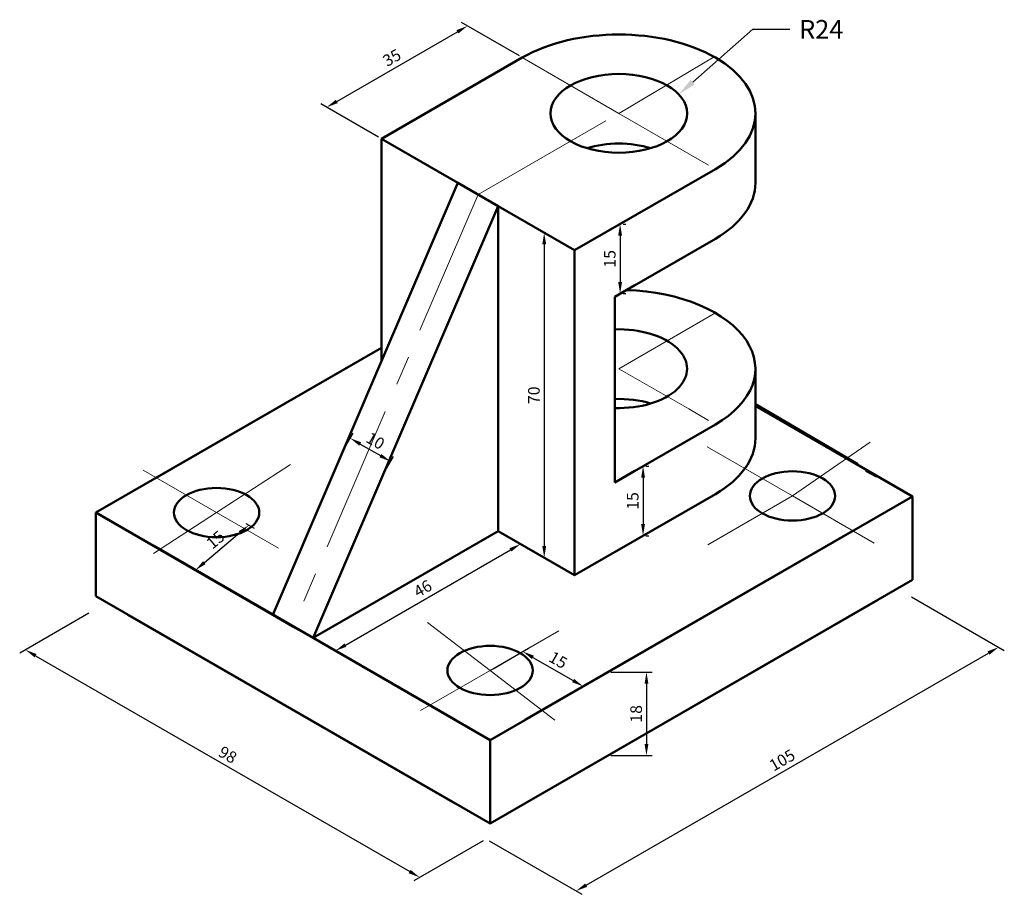
# Model space of a CAD drawing. Units: millimetres. Extents: x 3049 to 3261, y 1454 to 1642.
import ezdxf
from ezdxf import colors
from ezdxf.entities.mleader import LeaderData, LeaderLine
from ezdxf.math import Vec2, Vec3

# ---------------------------------------------------------------- set-up
doc = ezdxf.new("R2010")
doc.units = ezdxf.units.MM
doc.linetypes.add('CENTER', pattern=[50.8, 31.75, -6.35, 6.35, -6.35])
for name, color, linetype, lineweight in [('M-CNTR', 4, 'CENTER', 18), ('M-DIMS', 2, 'Continuous', 25), ('M-OUTL', 7, 'Continuous', 50)]:
    doc.layers.add(name, color=color, linetype=linetype, lineweight=lineweight)
doc.styles.get("Standard").update_dxf_attribs({"font": 'arial.ttf'})
doc.dimstyles.new('ISO-25', dxfattribs={"dimtxt": 2.5, "dimasz": 2.5, "dimexe": 1.25, "dimexo": 0.625, "dimtad": 1, "dimtxsty": 'Standard', "dimcen": 2.5, "dimadec": 0, "dimazin": 0, "dimtfac": 1, "dimtmove": 0, "dimatfit": 3, "dimfxl": 1, "dimarcsym": 0})

# ---------------------------------------------------------------- blocks, each defined once
blk = doc.blocks.new('*D1')
at = {"layer": 'Defpoints', "color": 0, "transparency": 16777216}
for p in [(3240.3, 1518.12), (3259.67, 1506.94), (3149.37, 1465.62)]:
    blk.add_point(p, dxfattribs=at)
at = {"layer": 'M-DIMS', "color": 0, "lineweight": -2, "transparency": 16777216}
for p, q in [((3240.93, 1517.76), (3260.92, 1506.22)), ((3170.91, 1455.69), (3257.51, 1505.69)), ((3149.99, 1465.26), (3169.99, 1453.72))]:
    blk.add_line(p, q, dxfattribs=at)
at = {"layer": 'M-DIMS', "color": 0, "transparency": 16777216}
for points in [[(3257.3, 1506.05), (3257.72, 1505.33), (3259.67, 1506.94)], [(3170.7, 1456.05), (3171.11, 1455.33), (3168.74, 1454.44)]]:
    blk.add_solid(points, dxfattribs=at)
at = {"layer": 'M-DIMS', "color": 0, "transparency": 16777216, "insert": (3213.26, 1482.34), "char_height": 2.5, "attachment_point": 5, "rotation": 30}
blk.add_mtext('105', dxfattribs=at)
blk = doc.blocks.new('*D2')
at = {"layer": 'Defpoints', "color": 0, "transparency": 16777216}
for p in [(3064.5, 1514.62), (3149.37, 1465.62), (3135.07, 1457.37)]:
    blk.add_point(p, dxfattribs=at)
at = {"layer": 'M-DIMS', "color": 0, "lineweight": -2, "transparency": 16777216}
for p, q in [((3063.87, 1514.26), (3048.95, 1505.65)), ((3052.37, 1505.12), (3132.91, 1458.62)), ((3148.74, 1465.26), (3133.82, 1456.65))]:
    blk.add_line(p, q, dxfattribs=at)
at = {"layer": 'M-DIMS', "color": 0, "transparency": 16777216}
for points in [[(3052.57, 1505.48), (3052.16, 1504.76), (3050.2, 1506.37)], [(3133.11, 1458.98), (3132.7, 1458.26), (3135.07, 1457.37)]]:
    blk.add_solid(points, dxfattribs=at)
at = {"layer": 'M-DIMS', "color": 0, "transparency": 16777216, "insert": (3093.59, 1483.51), "char_height": 2.5, "attachment_point": 5, "rotation": 330}
blk.add_mtext('98', dxfattribs=at)
blk = doc.blocks.new('*D3')
at = {"layer": 'Defpoints', "color": 0, "transparency": 16777216}
for p in [(3175.6, 1501.59), (3175.6, 1483.59), (3183.89, 1483.59)]:
    blk.add_point(p, dxfattribs=at)
at = {"layer": 'M-DIMS', "color": 0, "lineweight": -2, "transparency": 16777216}
for p, q in [((3176.23, 1501.59), (3185.14, 1501.59)), ((3183.89, 1499.09), (3183.89, 1486.09)), ((3176.23, 1483.59), (3185.14, 1483.59))]:
    blk.add_line(p, q, dxfattribs=at)
at = {"layer": 'M-DIMS', "color": 0, "transparency": 16777216}
for points in [[(3183.47, 1499.09), (3184.3, 1499.09), (3183.89, 1501.59)], [(3183.47, 1486.09), (3184.3, 1486.09), (3183.89, 1483.59)]]:
    blk.add_solid(points, dxfattribs=at)
at = {"layer": 'M-DIMS', "color": 0, "transparency": 16777216, "insert": (3181.99, 1492.59), "char_height": 2.5, "attachment_point": 5, "rotation": 90}
blk.add_mtext('18', dxfattribs=at)
blk = doc.blocks.new('*D4')
at = {"layer": 'Defpoints', "color": 0, "transparency": 16777216}
for p in [(3183.15, 1545.95), (3183.15, 1530.95), (3183.15, 1530.95)]:
    blk.add_point(p, dxfattribs=at)
at = {"layer": 'M-DIMS', "color": 0, "lineweight": -2, "transparency": 16777216}
for p, q in [((3183.78, 1545.95), (3184.4, 1545.95)), ((3183.15, 1543.45), (3183.15, 1533.45)), ((3183.78, 1530.95), (3184.4, 1530.95))]:
    blk.add_line(p, q, dxfattribs=at)
at = {"layer": 'M-DIMS', "color": 0, "transparency": 16777216}
for points in [[(3182.74, 1543.45), (3183.57, 1543.45), (3183.15, 1545.95)], [(3182.74, 1533.45), (3183.57, 1533.45), (3183.15, 1530.95)]]:
    blk.add_solid(points, dxfattribs=at)
at = {"layer": 'M-DIMS', "color": 0, "transparency": 16777216, "insert": (3181.25, 1538.45), "char_height": 2.5, "attachment_point": 5, "rotation": 90}
blk.add_mtext('15', dxfattribs=at)
blk = doc.blocks.new('*D5')
at = {"layer": 'Defpoints', "color": 0, "transparency": 16777216}
for p in [(3151.95, 1531.94), (3156.76, 1529.16), (3112.12, 1508.94)]:
    blk.add_point(p, dxfattribs=at)
at = {"layer": 'M-DIMS', "color": 0, "lineweight": -2, "transparency": 16777216}
for p, q in [((3152.58, 1531.57), (3158.01, 1528.44)), ((3119.09, 1507.41), (3154.6, 1527.91)), ((3112.74, 1508.57), (3118.18, 1505.44))]:
    blk.add_line(p, q, dxfattribs=at)
at = {"layer": 'M-DIMS', "color": 0, "transparency": 16777216}
for points in [[(3154.39, 1528.27), (3154.81, 1527.55), (3156.76, 1529.16)], [(3118.88, 1507.77), (3119.3, 1507.05), (3116.93, 1506.16)]]:
    blk.add_solid(points, dxfattribs=at)
at = {"layer": 'M-DIMS', "color": 0, "transparency": 16777216, "insert": (3135.89, 1519.31), "char_height": 2.5, "attachment_point": 5, "rotation": 30}
blk.add_mtext('46', dxfattribs=at)
blk = doc.blocks.new('*D6')
at = {"layer": 'Defpoints', "color": 0, "transparency": 16777216}
for p in [(3118.71, 1549.55), (3128.77, 1546.96), (3127.37, 1544.55)]:
    blk.add_point(p, dxfattribs=at)
at = {"layer": 'M-DIMS', "color": 0, "lineweight": -2, "transparency": 16777216}
for p, q in [((3119.02, 1550.09), (3120.73, 1553.04)), ((3122.27, 1550.71), (3126.6, 1548.21)), ((3127.68, 1545.09), (3129.39, 1548.04))]:
    blk.add_line(p, q, dxfattribs=at)
at = {"layer": 'M-DIMS', "color": 0, "transparency": 16777216}
for points in [[(3122.48, 1551.07), (3122.06, 1550.35), (3120.1, 1551.96)], [(3126.81, 1548.57), (3126.39, 1547.85), (3128.77, 1546.96)]]:
    blk.add_solid(points, dxfattribs=at)
at = {"layer": 'M-DIMS', "color": 0, "transparency": 16777216, "insert": (3125.39, 1551.11), "char_height": 2.5, "attachment_point": 5, "rotation": 330}
blk.add_mtext('10', dxfattribs=at)
blk = doc.blocks.new('*D7')
at = {"layer": 'Defpoints', "color": 0, "transparency": 16777216}
for p in [(3151.95, 1601.94), (3151.95, 1531.94), (3161.87, 1526.21)]:
    blk.add_point(p, dxfattribs=at)
at = {"layer": 'M-DIMS', "color": 0, "lineweight": -2, "transparency": 16777216}
for p, q in [((3152.58, 1601.57), (3163.12, 1595.49)), ((3161.87, 1593.71), (3161.87, 1528.71)), ((3152.58, 1531.57), (3163.12, 1525.49))]:
    blk.add_line(p, q, dxfattribs=at)
at = {"layer": 'M-DIMS', "color": 0, "transparency": 16777216}
for points in [[(3161.46, 1593.71), (3162.29, 1593.71), (3161.87, 1596.21)], [(3161.46, 1528.71), (3162.29, 1528.71), (3161.87, 1526.21)]]:
    blk.add_solid(points, dxfattribs=at)
at = {"layer": 'M-DIMS', "color": 0, "transparency": 16777216, "insert": (3159.97, 1561.21), "char_height": 2.5, "attachment_point": 5, "rotation": 90}
blk.add_mtext('70', dxfattribs=at)
blk = doc.blocks.new('*D8')
at = {"layer": 'Defpoints', "color": 0, "transparency": 16777216}
for p in [(3145.35, 1640.75), (3157.15, 1633.94), (3126.84, 1616.44)]:
    blk.add_point(p, dxfattribs=at)
at = {"layer": 'M-DIMS', "color": 0, "lineweight": -2, "transparency": 16777216}
for p, q in [((3156.53, 1634.3), (3144.1, 1641.47)), ((3117.21, 1624.5), (3143.19, 1639.5)), ((3126.22, 1616.8), (3113.79, 1623.97))]:
    blk.add_line(p, q, dxfattribs=at)
at = {"layer": 'M-DIMS', "color": 0, "transparency": 16777216}
for points in [[(3142.98, 1639.86), (3143.39, 1639.14), (3145.35, 1640.75)], [(3117, 1624.86), (3117.41, 1624.14), (3115.04, 1623.25)]]:
    blk.add_solid(points, dxfattribs=at)
at = {"layer": 'M-DIMS', "color": 0, "transparency": 16777216, "insert": (3129.24, 1633.65), "char_height": 2.5, "attachment_point": 5, "rotation": 30}
blk.add_mtext('35', dxfattribs=at)
blk = doc.blocks.new('*D9')
at = {"layer": 'Defpoints', "color": 0, "transparency": 16777216}
for p in [(3150.22, 1501.94), (3170.26, 1498.51), (3163.21, 1494.44)]:
    blk.add_point(p, dxfattribs=at)
at = {"layer": 'M-DIMS', "color": 0, "lineweight": -2, "transparency": 16777216}
for p, q in [((3150.85, 1502.3), (3158.52, 1506.73)), ((3159.44, 1504.76), (3168.1, 1499.76)), ((3163.84, 1494.8), (3171.51, 1499.23))]:
    blk.add_line(p, q, dxfattribs=at)
at = {"layer": 'M-DIMS', "color": 0, "transparency": 16777216}
for points in [[(3159.65, 1505.12), (3159.23, 1504.39), (3157.27, 1506.01)], [(3168.31, 1500.12), (3167.89, 1499.39), (3170.26, 1498.51)]]:
    blk.add_solid(points, dxfattribs=at)
at = {"layer": 'M-DIMS', "color": 0, "transparency": 16777216, "insert": (3164.72, 1503.9), "char_height": 2.5, "attachment_point": 5, "rotation": 330}
blk.add_mtext('15', dxfattribs=at)
blk = doc.blocks.new('*D10')
at = {"layer": 'Defpoints', "color": 0, "transparency": 16777216}
for p in [(3097.06, 1533.92), (3098.26, 1533.23), (3085.59, 1524.25)]:
    blk.add_point(p, dxfattribs=at)
at = {"layer": 'M-DIMS', "color": 0, "lineweight": -2, "transparency": 16777216}
for p, q in [((3097.63, 1533.59), (3099.41, 1532.56)), ((3088.71, 1525.17), (3096.35, 1531.62)), ((3086.17, 1523.92), (3087.95, 1522.89))]:
    blk.add_line(p, q, dxfattribs=at)
at = {"layer": 'M-DIMS', "color": 0, "transparency": 16777216}
for points in [[(3096.08, 1531.93), (3096.62, 1531.3), (3098.26, 1533.23)], [(3088.44, 1525.48), (3088.98, 1524.85), (3086.8, 1523.55)]]:
    blk.add_solid(points, dxfattribs=at)
at = {"layer": 'M-DIMS', "color": 0, "transparency": 16777216, "insert": (3091.3, 1529.84), "char_height": 2.5, "attachment_point": 5, "rotation": 40.1597}
blk.add_mtext('15', dxfattribs=at)
blk = doc.blocks.new('*D11')
at = {"layer": 'Defpoints', "color": 0, "transparency": 16777216}
for p in [(3178.21, 1598.1), (3178.21, 1583.1), (3178.21, 1583.1)]:
    blk.add_point(p, dxfattribs=at)
at = {"layer": 'M-DIMS', "color": 0, "lineweight": -2, "transparency": 16777216}
for p, q in [((3178.84, 1598.1), (3179.46, 1598.1)), ((3178.21, 1595.6), (3178.21, 1585.6)), ((3178.84, 1583.1), (3179.46, 1583.1))]:
    blk.add_line(p, q, dxfattribs=at)
at = {"layer": 'M-DIMS', "color": 0, "transparency": 16777216}
for points in [[(3177.8, 1595.6), (3178.63, 1595.6), (3178.21, 1598.1)], [(3177.8, 1585.6), (3178.63, 1585.6), (3178.21, 1583.1)]]:
    blk.add_solid(points, dxfattribs=at)
at = {"layer": 'M-DIMS', "color": 0, "transparency": 16777216, "insert": (3176.31, 1590.6), "char_height": 2.5, "attachment_point": 5, "rotation": 90}
blk.add_mtext('15', dxfattribs=at)

msp = doc.modelspace()

# ---------------------------------------------------------------- linework, layer by layer
at = {"layer": 'M-CNTR'}
for p, q in [((3177.936, 1621.936), (3157.151, 1633.936)), ((3177.936, 1621.936), (3198.452, 1634.088)), ((3147.625, 1604.436), (3177.936, 1621.936)), ((3177.936, 1621.936), (3197.27, 1610.773)), ((3147.625, 1604.436), (3107.788, 1511.436)), ((3177.936, 1566.936), (3198.72, 1578.936)), ((3177.936, 1566.936), (3192.972, 1558.254)), ((3192.972, 1558.254), (3197.216, 1555.804)), ((3215.326, 1539.523), (3196.963, 1550.125)), ((3215.326, 1539.523), (3232.078, 1551.142)), ((3091.333, 1535.936), (3107.263, 1546.286)), ((3091.333, 1535.936), (3075.561, 1545.042)), ((3215.326, 1539.523), (3197.062, 1528.978)), ((3215.326, 1539.523), (3232.911, 1529.371)), ((3091.333, 1535.936), (3077.724, 1527.093)), ((3091.333, 1535.936), (3104.654, 1528.245)), ((3150.223, 1501.936), (3136.735, 1512.301)), ((3150.223, 1501.936), (3164.985, 1510.458)), ((3150.223, 1501.936), (3158.976, 1506.989)), ((3150.223, 1501.936), (3135.254, 1493.293)), ((3150.223, 1501.936), (3164.126, 1491.251))]:
    msp.add_line(p, q, dxfattribs=at)
at = {"layer": 'M-OUTL'}
for p, q in [((3157.151, 1633.936), (3126.84, 1616.436)), ((3207.329, 1606.936), (3207.329, 1621.936)), ((3143.295, 1606.936), (3126.84, 1616.436)), ((3126.84, 1616.436), (3126.84, 1568.523)), ((3198.72, 1609.936), (3168.409, 1592.436)), ((3103.457, 1513.936), (3143.295, 1606.936)), ((3147.625, 1604.436), (3143.295, 1606.936)), ((3143.295, 1606.936), (3151.955, 1601.936)), ((3112.118, 1508.936), (3151.955, 1601.936)), ((3151.955, 1601.936), (3168.409, 1592.436)), ((3151.955, 1601.936), (3151.955, 1531.936)), ((3168.409, 1592.436), (3181.4, 1599.936)), ((3198.72, 1594.936), (3177.07, 1582.436)), ((3168.409, 1592.436), (3168.409, 1522.436)), ((3177.07, 1582.436), (3181.4, 1584.936)), ((3177.07, 1582.436), (3181.4, 1584.936)), ((3177.07, 1582.436), (3177.07, 1542.436)), ((3065.349, 1535.936), (3126.837, 1571.436)), ((3078.343, 1543.436), (3126.84, 1571.436)), ((3207.329, 1551.936), (3207.329, 1566.936)), ((3241.152, 1539.436), (3207.326, 1558.965)), ((3229.362, 1546.366), (3207.329, 1559.315)), ((3198.72, 1554.936), (3177.07, 1542.436)), ((3177.07, 1542.436), (3181.4, 1544.936)), ((3233.376, 1543.708), (3231.106, 1544.955)), ((3150.219, 1486.936), (3241.152, 1539.436)), ((3198.72, 1539.936), (3168.409, 1522.436)), ((3241.152, 1521.436), (3241.152, 1539.436)), ((3103.454, 1513.936), (3065.349, 1535.936)), ((3065.349, 1517.936), (3065.349, 1535.936)), ((3112.118, 1508.936), (3151.955, 1531.936)), ((3151.955, 1531.936), (3168.409, 1522.436)), ((3157.723, 1491.266), (3228.317, 1532.023)), ((3241.155, 1530.096), (3241.155, 1530.56)), ((3077.807, 1528.758), (3077.8, 1528.749)), ((3142.723, 1491.266), (3077.8, 1528.749)), ((3181.4, 1529.936), (3168.409, 1522.436)), ((3168.409, 1522.436), (3181.4, 1529.936)), ((3150.219, 1468.936), (3241.152, 1521.436)), ((3150.219, 1468.936), (3065.349, 1517.936)), ((3157.723, 1473.266), (3233.655, 1517.105)), ((3072.264, 1513.945), (3142.723, 1473.266)), ((3107.788, 1511.436), (3103.457, 1513.936)), ((3107.788, 1511.436), (3112.118, 1508.936)), ((3150.219, 1486.936), (3112.114, 1508.936)), ((3150.219, 1468.936), (3150.219, 1486.936))]:
    msp.add_line(p, q, dxfattribs=at)
for centre, major_axis, start_param, end_param in [((3177.936, 1621.936), (-29.394, 0), 2.3561945, 5.4977871), ((3177.932, 1606.936), (14.697, 0), 1.0841014, 2.0574913), ((3177.936, 1606.936), (-29.394, 0), 2.3561945, 3.1415927), ((3177.936, 1566.936), (-29.394, 0), 2.3561945, 4.6567185), ((3177.936, 1566.936), (-14.697, 0), 1.5118366, 4.7713487), ((3177.932, 1551.936), (14.697, 0), 1.0841014, 1.629756), ((3177.936, 1551.936), (-29.394, 0), 2.3561945, 3.1415927)]:
    msp.add_ellipse(centre, major_axis=major_axis, ratio=0.5773503, start_param=start_param, end_param=end_param, dxfattribs=at)
for centre, major_axis in [((3177.936, 1621.936), (-14.697, 0)), ((3215.326, 1539.523), (-9.186, 0)), ((3091.333, 1535.936), (-9.186, 0)), ((3150.223, 1501.936), (-9.186, 0))]:
    msp.add_ellipse(centre, major_axis=major_axis, ratio=0.5773503, dxfattribs=at)

# ---------------------------------------------------------------- dimensions: what is measured, and where the dimension line sits
at = {"layer": 'M-DIMS'}
for p1, p2, distance, picture, middle in [((3126.84, 1616.436), (3157.151, 1633.936), 11.799, '*D8', (3129.245, 1633.645)), ((3151.955, 1601.936), (3151.955, 1531.936), 9.918, '*D7', (3159.972, 1561.209)), ((3178.214, 1598.096), (3178.214, 1583.096), 0, '*D11', (3176.313, 1590.596)), ((3118.711, 1549.545), (3127.371, 1544.545), 2.788, '*D6', (3125.386, 1551.106)), ((3183.154, 1545.949), (3183.154, 1530.949), 0, '*D4', (3181.253, 1538.449)), ((3085.592, 1524.25), (3097.056, 1533.924), -1.31, '*D10', (3091.304, 1529.844)), ((3112.118, 1508.936), (3151.955, 1531.936), -4.809, '*D5', (3135.894, 1519.306)), ((3149.37, 1465.623), (3240.303, 1518.123), -19.37, '*D1', (3213.256, 1482.336)), ((3064.499, 1514.623), (3149.37, 1465.623), -14.299, '*D2', (3093.587, 1483.514)), ((3150.223, 1501.936), (3163.213, 1494.436), 7.049, '*D9', (3164.718, 1503.902)), ((3175.601, 1501.588), (3175.601, 1483.588), 8.286, '*D3', (3181.985, 1492.588))]:
    dim = msp.add_aligned_dim(p1=p1, p2=p2, distance=distance, dimstyle='ISO-25', override={"dimclrd": 0, "dimclre": 0, "dimclrt": 0}, dxfattribs=at)
    dim.commit()
    dim.dimension.update_dxf_attribs({"geometry": picture, "text_midpoint": middle})

# ---------------------------------------------------------------- leaders
ml = msp.add_multileader_mtext('Standard', dxfattribs=at)
ml.set_content('R24', color=256)
ml.set_leader_properties()
ml.build(insert=Vec2(0, 0))
ctx = ml.context
ctx.base_point, ctx.plane_origin = Vec3(3214.751, 1640.039), Vec3(3190.833, 1626.004)
notes = []
notes.append((ctx, [(0, (1, 1, 0), (3206.751, 1640.039), (1, 0), 8, [(0, [(3190.833, 1626.004)], 0, [])])]))
ctx.mtext.insert, ctx.mtext.flow_direction = Vec3(3216.751, 1642.039), 5
for ctx, leaders in notes:
    for number, flags, end, landing, length, lines in leaders:
        leader = LeaderData()
        leader.index, (leader.has_last_leader_line, leader.has_dogleg_vector, leader.attachment_direction) = number, flags
        leader.last_leader_point, leader.dogleg_vector, leader.dogleg_length = Vec3(end), Vec3(landing), length
        for number, points, colour, breaks in lines:
            line = LeaderLine()
            line.index, line.vertices, line.color, line.breaks = number, Vec3.list(points), colors.encode_raw_color(colour), breaks
            leader.lines.append(line)
        ctx.leaders.append(leader)

doc.saveas('drawing.dxf')
